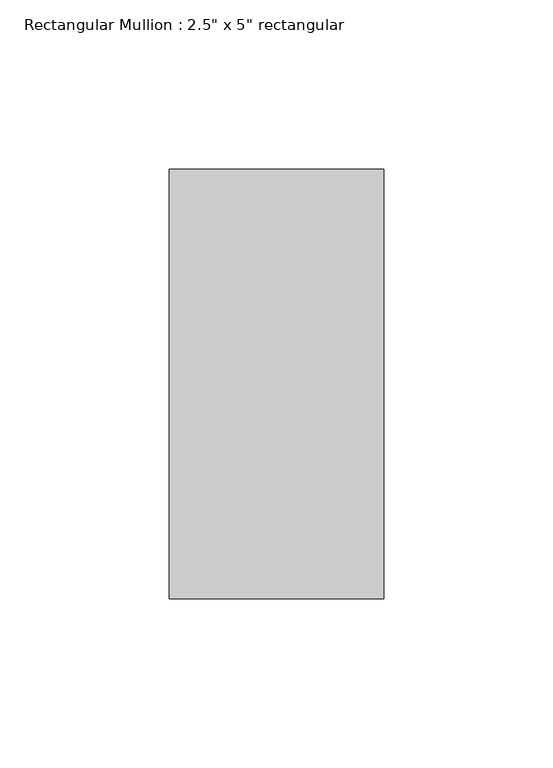
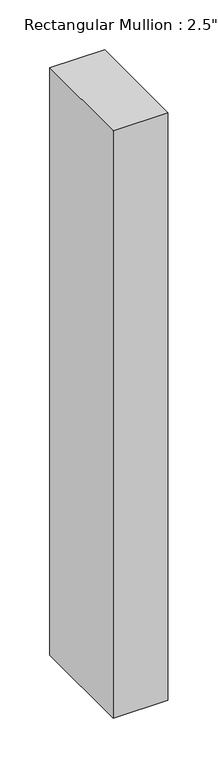
"""IFC4 building model written with IfcOpenShell, lengths in millimetres: member geometry."""

from ifc_helpers import new_model, si_unit, frame, origin, place, context, project, spatial, polyline, outline, extrude, source, transform, mapped, element, save


def member_411778f3(model_context):
    return source(origin(), model_context, "Body", "SweptSolid", [
        extrude(outline(polyline([(0.0, 63.5), (0.0, -63.5), (-63.5, -63.5), (-63.5, 63.5), (0.0, 63.5)])), frame((0.0, 0.0, -719.6039078), z_axis=(0.0, 0.0, 1.0), x_axis=(1.0, 0.0, 0.0)), (0.0, 0.0, 1.0), 719.6039078),
    ])


if __name__ == "__main__":
    model = new_model("IFC4")
    model_context = context("Model", 3, world=origin())
    ifc_project = project(units=[si_unit("LENGTHUNIT", "METRE", prefix="MILLI")], contexts=[model_context])
    site = spatial("IfcSite", under=ifc_project)
    building = spatial("IfcBuilding", under=site)
    placement = place(None, origin())
    member_shape = member_411778f3(model_context)
    element("IfcMember", 1, ObjectType="Rectangular Mullion : 2.5\" x 5\" rectangular", at=placement, inside=building, context=model_context, shape_type="MappedRepresentation", body=[
        mapped(member_shape, transform((0.0, 0.0, 0.0), x_axis=(1.0, 0.0, 0.0), y_axis=(0.0, 1.0, 0.0), z_axis=(0.0, 0.0, 1.0))),
    ])
    save(model, "model.ifc")

# Revit data of these elements
# Type "Rectangular Mullion : 2.5\" x 5\" rectangular"
#   built-in parameter 1007304 = 0.416667 (stored number, unit not read)
#   built-in parameter 1007301 = 0.104167 (stored number, unit not read)
#   built-in parameter 1007300 = 0.104167 (stored number, unit not read)
# Element 1 (IfcMember, "Rectangular Mullion : 2.5\" x 5\" rectangular")
#   Materials on its faces: "Aluminum"
# Materials
#   "Aluminum": class "Metal", colour RGB 247 247 247, transparency 0, Description = "Aluminum 6061", Cost = 0
